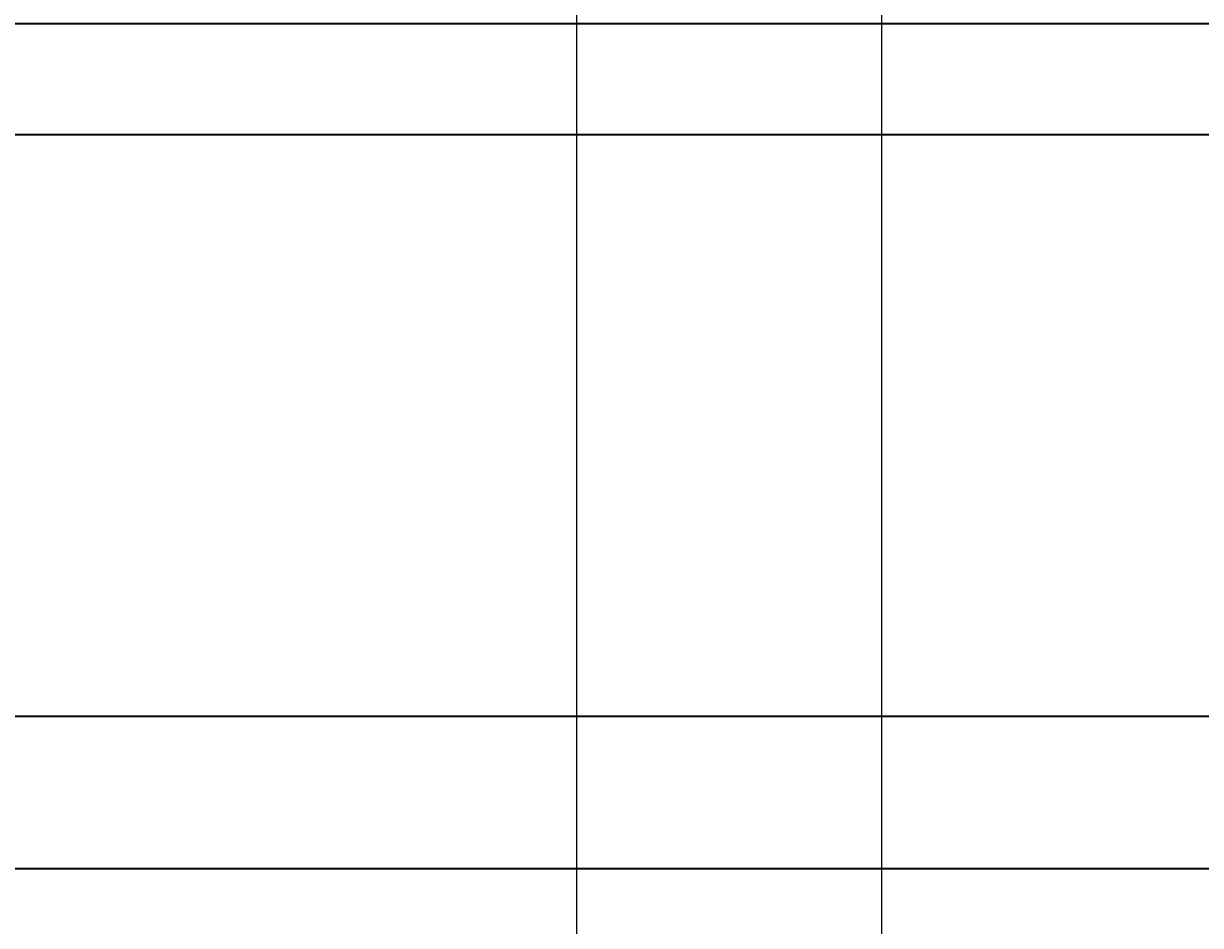
# Model space of a CAD drawing. Units: inches. Extents: x -6 to 289, y -8 to 323.
# Tile 101 of 107: x 219 to 243, y 276 to 294. Entities that reach past the tile are written whole.
import ezdxf

# ---------------------------------------------------------------- set-up
doc = ezdxf.new("R2010")
doc.units = ezdxf.units.IN
doc.header["$MEASUREMENT"] = 0
doc.layers.add('A-ANNO-DIMS', color=2, linetype='Continuous', lineweight=18)
doc.layers.add('A-ELEV', color=7, linetype='Continuous', lineweight=35)
doc.styles.get("Standard").update_dxf_attribs({"font": 'arial.ttf'})
doc.dimstyles.get("Standard").update_dxf_attribs({"dimtxt": 0.18, "dimasz": 0.18, "dimexe": 0.18, "dimexo": 0.0625, "dimgap": 0.09, "dimtad": 0, "dimtih": 1, "dimtoh": 1, "dimdec": 4, "dimzin": 0, "dimdsep": 46, "dimtxsty": 'Standard', "dimcen": 0.09, "dimadec": 0, "dimazin": 0, "dimtfac": 1, "dimtdec": 4, "dimtofl": 0, "dimtmove": 0, "dimatfit": 3, "dimfxl": 1, "dimtolj": 1, "dimtzin": 0, "dimarcsym": 0})

# ---------------------------------------------------------------- blocks, each defined once
blk = doc.blocks.new('*D13')
at = {"layer": 'A-ANNO-DIMS', "color": 0, "lineweight": -2, "transparency": 16777216}
for p, q in [((188.292, 226.951), (188.292, 322.969)), ((236.292, 226.951), (236.292, 322.969)), ((188.472, 322.789), (212.069, 322.789)), ((236.112, 322.789), (212.515, 322.789))]:
    blk.add_line(p, q, dxfattribs=at)
at = {"layer": 'A-ANNO-DIMS', "color": 0, "transparency": 16777216}
for points in [[(188.472, 322.819), (188.472, 322.759), (188.292, 322.789)], [(236.112, 322.819), (236.112, 322.759), (236.292, 322.789)]]:
    blk.add_solid(points, dxfattribs=at)
at = {"layer": 'Defpoints', "color": 0, "transparency": 16777216}
for p in [(236.292, 322.789), (188.292, 226.889), (236.292, 226.889)]:
    blk.add_point(p, dxfattribs=at)
at = {"layer": 'A-ANNO-DIMS', "color": 0, "transparency": 16777216, "insert": (212.292, 322.789), "char_height": 0.18, "attachment_point": 5}
blk.add_mtext('\\A1;48', dxfattribs=at)
blk = doc.blocks.new('*D14')
at = {"layer": 'A-ANNO-DIMS', "color": 0, "lineweight": -2, "transparency": 16777216}
for p, q in [((236.292, 226.951), (236.292, 322.969)), ((247.164, 162.411), (247.164, 322.969)), ((236.472, 322.789), (241.274, 322.789)), ((246.984, 322.789), (242.182, 322.789))]:
    blk.add_line(p, q, dxfattribs=at)
at = {"layer": 'A-ANNO-DIMS', "color": 0, "transparency": 16777216}
for points in [[(236.472, 322.819), (236.472, 322.759), (236.292, 322.789)], [(246.984, 322.819), (246.984, 322.759), (247.164, 322.789)]]:
    blk.add_solid(points, dxfattribs=at)
at = {"layer": 'Defpoints', "color": 0, "transparency": 16777216}
for p in [(247.164, 322.789), (236.292, 226.889), (247.164, 162.348)]:
    blk.add_point(p, dxfattribs=at)
at = {"layer": 'A-ANNO-DIMS', "color": 0, "transparency": 16777216, "insert": (241.728, 322.789), "char_height": 0.18, "attachment_point": 5}
blk.add_mtext('\\A1;10.872', dxfattribs=at)
blk = doc.blocks.new('*D27')
at = {"layer": 'A-ANNO-DIMS', "color": 0, "lineweight": -2, "transparency": 16777216}
for p, q in [((19.226, 307.289), (288.653, 307.289)), ((288.473, 307.109), (288.473, 277.471)), ((288.473, 247.469), (288.473, 277.107)), ((247.226, 247.289), (288.653, 247.289))]:
    blk.add_line(p, q, dxfattribs=at)
at = {"layer": 'A-ANNO-DIMS', "color": 0, "transparency": 16777216}
for points in [[(288.443, 307.109), (288.503, 307.109), (288.473, 307.289)], [(288.443, 247.469), (288.503, 247.469), (288.473, 247.289)]]:
    blk.add_solid(points, dxfattribs=at)
at = {"layer": 'Defpoints', "color": 0, "transparency": 16777216}
for p in [(19.164, 307.289), (288.473, 307.289), (247.164, 247.289)]:
    blk.add_point(p, dxfattribs=at)
at = {"layer": 'A-ANNO-DIMS', "color": 0, "transparency": 16777216, "insert": (288.473, 277.289), "char_height": 0.18, "attachment_point": 5}
blk.add_mtext('\\A1;60', dxfattribs=at)
blk = doc.blocks.new('*D80')
at = {"layer": 'A-ANNO-DIMS', "color": 0, "lineweight": -2, "transparency": 16777216}
for p, q in [((188.292, 116.842), (188.292, 322.969)), ((230.292, 116.842), (230.292, 322.969)), ((188.472, 322.789), (209.07, 322.789)), ((230.112, 322.789), (209.513, 322.789))]:
    blk.add_line(p, q, dxfattribs=at)
at = {"layer": 'A-ANNO-DIMS', "color": 0, "transparency": 16777216}
for points in [[(188.472, 322.819), (188.472, 322.759), (188.292, 322.789)], [(230.112, 322.819), (230.112, 322.759), (230.292, 322.789)]]:
    blk.add_solid(points, dxfattribs=at)
at = {"layer": 'Defpoints', "color": 0, "transparency": 16777216}
for p in [(230.292, 322.789), (188.292, 116.779), (230.292, 116.779)]:
    blk.add_point(p, dxfattribs=at)
at = {"layer": 'A-ANNO-DIMS', "color": 0, "transparency": 16777216, "insert": (209.292, 322.789), "char_height": 0.18, "attachment_point": 5}
blk.add_mtext('\\A1;42', dxfattribs=at)
blk = doc.blocks.new('*D81')
at = {"layer": 'A-ANNO-DIMS', "color": 0, "lineweight": -2, "transparency": 16777216}
for p, q in [((230.292, 68.842), (230.292, 322.969)), ((245.215, 66.286), (245.215, 322.969)), ((230.472, 322.789), (237.298, 322.789)), ((245.035, 322.789), (238.208, 322.789))]:
    blk.add_line(p, q, dxfattribs=at)
at = {"layer": 'A-ANNO-DIMS', "color": 0, "transparency": 16777216}
for points in [[(230.472, 322.819), (230.472, 322.759), (230.292, 322.789)], [(245.035, 322.819), (245.035, 322.759), (245.215, 322.789)]]:
    blk.add_solid(points, dxfattribs=at)
at = {"layer": 'Defpoints', "color": 0, "transparency": 16777216}
for p in [(245.215, 322.789), (230.292, 68.779), (245.215, 66.224)]:
    blk.add_point(p, dxfattribs=at)
at = {"layer": 'A-ANNO-DIMS', "color": 0, "transparency": 16777216, "insert": (237.753, 322.789), "char_height": 0.18, "attachment_point": 5}
blk.add_mtext('\\A1;14.923', dxfattribs=at)
blk = doc.blocks.new('*D98')
at = {"layer": 'A-ANNO-DIMS', "color": 0, "lineweight": -2, "transparency": 16777216}
for p, q in [((202.741, 159.411), (202.741, 322.969)), ((244.164, 159.411), (244.164, 322.969)), ((202.921, 322.789), (223.056, 322.789)), ((243.984, 322.789), (223.849, 322.789))]:
    blk.add_line(p, q, dxfattribs=at)
at = {"layer": 'A-ANNO-DIMS', "color": 0, "transparency": 16777216}
for points in [[(202.921, 322.819), (202.921, 322.759), (202.741, 322.789)], [(243.984, 322.819), (243.984, 322.759), (244.164, 322.789)]]:
    blk.add_solid(points, dxfattribs=at)
at = {"layer": 'Defpoints', "color": 0, "transparency": 16777216}
for p in [(244.164, 322.789), (202.741, 159.348), (244.164, 159.348)]:
    blk.add_point(p, dxfattribs=at)
at = {"layer": 'A-ANNO-DIMS', "color": 0, "transparency": 16777216, "insert": (223.452, 322.789), "char_height": 0.18, "attachment_point": 5}
blk.add_mtext('\\A1;41.42', dxfattribs=at)
blk = doc.blocks.new('*D108')
at = {"layer": 'A-ANNO-DIMS', "color": 0, "lineweight": -2, "transparency": 16777216}
for p, q in [((186.984, 291.541), (186.984, 322.969)), ((255.804, 291.541), (255.804, 322.969)), ((187.164, 322.789), (221, 322.789)), ((255.624, 322.789), (221.787, 322.789))]:
    blk.add_line(p, q, dxfattribs=at)
at = {"layer": 'A-ANNO-DIMS', "color": 0, "transparency": 16777216}
for points in [[(187.164, 322.819), (187.164, 322.759), (186.984, 322.789)], [(255.624, 322.819), (255.624, 322.759), (255.804, 322.789)]]:
    blk.add_solid(points, dxfattribs=at)
at = {"layer": 'Defpoints', "color": 0, "transparency": 16777216}
for p in [(255.804, 322.789), (186.984, 291.478), (255.804, 291.478)]:
    blk.add_point(p, dxfattribs=at)
at = {"layer": 'A-ANNO-DIMS', "color": 0, "transparency": 16777216, "insert": (221.394, 322.789), "char_height": 0.18, "attachment_point": 5}
blk.add_mtext('\\A1;68.82', dxfattribs=at)

msp = doc.modelspace()

# ---------------------------------------------------------------- linework, layer by layer
at = {"layer": 'A-ELEV'}
for points in [[(115.1638, 307.2888), (115.1638, 277.0427), (259.1638, 277.0427), (259.1638, 259.2888)], [(118.1638, 307.2888), (118.1638, 280.0427), (262.1638, 280.0427), (262.1638, 259.2888)], [(255.8036, 291.4781), (118.1638, 291.4781), (118.1638, 293.6657), (255.8036, 293.6657)]]:
    msp.add_lwpolyline(points, dxfattribs=at)

# ---------------------------------------------------------------- dimensions: what is measured, and where the dimension line sits
at = {"layer": 'A-ANNO-DIMS'}
for base, p1, p2, override, picture, middle in [((255.8036, 322.7888), (186.9837, 291.4781), (255.8036, 291.4781), {"dimdec": 2, "dimlfac": 1, "dimrnd": 0, "dimzin": 0, "dimdsep": 46, "dimlunit": 2}, '*D108', (221.3936, 322.7888)), ((236.2918, 322.7888), (188.2918, 226.8887), (236.2918, 226.8887), {"dimdec": 0, "dimlfac": 1, "dimrnd": 0, "dimzin": 0, "dimdsep": 46, "dimlunit": 2}, '*D13', (212.2918, 322.7888)), ((230.2918, 322.7888), (188.2918, 116.7795), (230.2918, 116.7795), {"dimdec": 0, "dimlfac": 1, "dimrnd": 0, "dimzin": 0, "dimdsep": 46, "dimlunit": 2}, '*D80', (209.2918, 322.7888)), ((244.1638, 322.7888), (202.741, 159.3484), (244.1638, 159.3484), {"dimdec": 2, "dimlfac": 1, "dimrnd": 0, "dimzin": 0, "dimdsep": 46, "dimlunit": 2}, '*D98', (223.4524, 322.7888)), ((245.2146, 322.7888), (230.2918, 68.7795), (245.2146, 66.2238), {"dimdec": 3, "dimlfac": 1, "dimrnd": 0, "dimzin": 0, "dimdsep": 46, "dimlunit": 2}, '*D81', (237.7532, 322.7888)), ((247.1638, 322.7888), (236.2918, 226.8887), (247.1638, 162.3484), {"dimdec": 3, "dimlfac": 1, "dimrnd": 0, "dimzin": 0, "dimdsep": 46, "dimlunit": 2}, '*D14', (241.7278, 322.7888))]:
    dim = msp.add_linear_dim(base=base, p1=p1, p2=p2, dimstyle='Standard', override=override, dxfattribs=at)
    dim.commit()
    dim.dimension.update_dxf_attribs({"geometry": picture, "text_midpoint": middle})
dim = msp.add_linear_dim(base=(288.4733, 307.2888), p1=(247.1638, 247.2888), p2=(19.1638, 307.2888), angle=90, dimstyle='Standard', override={"dimdec": 0, "dimlfac": 1, "dimrnd": 0, "dimzin": 0, "dimdsep": 46, "dimlunit": 2}, dxfattribs=at)
dim.commit()
dim.dimension.update_dxf_attribs({"geometry": '*D27', "text_midpoint": (288.4733, 277.2888)})

doc.saveas('drawing.dxf')
